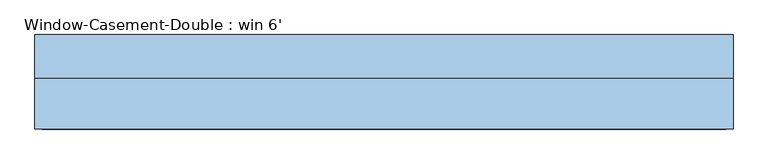
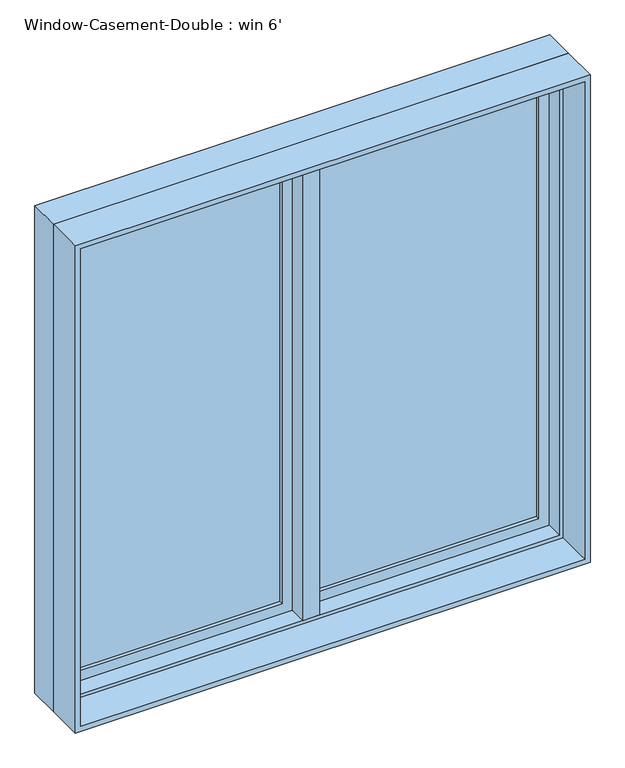
"""IFC4 building model written with IfcOpenShell, lengths in millimetres: window geometry, Window-Casement-Double : win 6'."""

from ifc_helpers import new_model, si_unit, frame, origin, place, context, project, spatial, polyline, outline, extrude, faceted_brep, source, transform, mapped, element, save


def window_casement_double_win_6_ce442eab(model_context):
    return source(origin(), model_context, "Body", "SolidModel", [
        faceted_brep([(9.525, 133.35, 2730.5), (-9.525, 133.35, 2730.5), (-9.525, 82.55, 2730.5), (9.525, 82.55, 2730.5), (9.525, 133.35, 927.1), (9.525, 82.55, 927.1), (-9.525, 82.55, 927.1), (-9.525, 133.35, 927.1), (-9.525, 82.55, 946.15), (-9.525, 82.55, 2711.45), (-30.1625, 82.55, 946.15), (-30.1625, 82.55, 2711.45), (-30.1625, 19.05, 946.15), (-30.1625, 19.05, 2711.45), (30.1625, 19.05, 946.15), (30.1625, 19.05, 2711.45), (30.1625, 82.55, 946.15), (30.1625, 82.55, 2711.45), (9.525, 82.55, 946.15), (9.525, 82.55, 2711.45)], [[[0, 1, 2, 3]], [[4, 5, 6, 7]], [[1, 0, 4, 7]], [[2, 1, 7, 6, 8, 9]], [[9, 8, 10, 11]], [[11, 10, 12, 13]], [[13, 12, 14, 15]], [[15, 14, 16, 17]], [[17, 16, 18, 19]], [[0, 3, 19, 18, 5, 4]], [[18, 8, 6, 5]], [[9, 19, 3, 2]], [[8, 18, 16, 14, 12, 10]], [[19, 9, 11, 13, 15, 17]]]),
        extrude(outline(polyline([(-66.675, 114.3), (-66.675, 107.95), (-844.55, 107.95), (-844.55, 114.3), (-66.675, 114.3)])), frame((0.0, 0.0, 984.25), z_axis=(0.0, 0.0, 1.0), x_axis=(1.0, 0.0, 0.0)), (0.0, 0.0, 1.0), 1689.1),
        extrude(outline(polyline([(-844.55, 95.25), (-844.55, 101.6), (-66.675, 101.6), (-66.675, 95.25), (-844.55, 95.25)])), frame((0.0, 0.0, 984.25), z_axis=(0.0, 0.0, 1.0), x_axis=(1.0, 0.0, 0.0)), (0.0, 0.0, 1.0), 1689.1),
        extrude(outline(polyline([(844.55, 114.3), (844.55, 107.95), (66.675, 107.95), (66.675, 114.3), (844.55, 114.3)])), frame((0.0, 0.0, 984.25), z_axis=(0.0, 0.0, 1.0), x_axis=(1.0, 0.0, 0.0)), (0.0, 0.0, 1.0), 1689.1),
        extrude(outline(polyline([(66.675, 95.25), (66.675, 101.6), (844.55, 101.6), (844.55, 95.25), (66.675, 95.25)])), frame((0.0, 0.0, 984.25), z_axis=(0.0, 0.0, 1.0), x_axis=(1.0, 0.0, 0.0)), (0.0, 0.0, 1.0), 1689.1),
        extrude(outline(polyline([(2730.5, -901.7), (927.1, -901.7), (927.1, -9.525), (2730.5, -9.525), (2730.5, -901.7)]), holes=[polyline([(2673.35, -66.675), (984.25, -66.675), (984.25, -844.55), (2673.35, -844.55), (2673.35, -66.675)])]), frame((0.0, 82.55, 0.0), z_axis=(0.0, 1.0, 0.0), x_axis=(0.0, 0.0, 1.0)), (0.0, 0.0, 1.0), 44.45),
        extrude(outline(polyline([(927.1, 901.7), (2730.5, 901.7), (2730.5, 9.525), (927.1, 9.525), (927.1, 901.7)]), holes=[polyline([(984.25, 66.675), (2673.35, 66.675), (2673.35, 844.55), (984.25, 844.55), (984.25, 66.675)])]), frame((0.0, 82.55, 0.0), z_axis=(0.0, 1.0, 0.0), x_axis=(0.0, 0.0, 1.0)), (0.0, 0.0, 1.0), 44.45),
        extrude(outline(polyline([(2743.2, -914.4), (914.4, -914.4), (914.4, 914.4), (2743.2, 914.4), (2743.2, -914.4)]), holes=[polyline([(2724.15, 895.35), (933.45, 895.35), (933.45, -895.35), (2724.15, -895.35), (2724.15, 895.35)])]), frame((0.0, -114.3, 0.0), z_axis=(0.0, 1.0, 0.0), x_axis=(0.0, 0.0, 1.0)), (0.0, 0.0, 1.0), 133.35),
        faceted_brep([(882.65, 82.55, 2711.45), (882.65, 19.05, 2711.45), (-882.65, 19.05, 2711.45), (-882.65, 82.55, 2711.45), (901.7, 133.35, 2730.5), (901.7, 82.55, 2730.5), (-901.7, 82.55, 2730.5), (-901.7, 133.35, 2730.5), (914.4, 19.05, 2743.2), (914.4, 133.35, 2743.2), (-914.4, 133.35, 2743.2), (-914.4, 19.05, 2743.2), (-882.65, 19.05, 946.15), (-882.65, 82.55, 946.15), (-901.7, 82.55, 927.1), (-901.7, 133.35, 927.1), (-914.4, 133.35, 914.4), (-914.4, 19.05, 914.4), (882.65, 19.05, 946.15), (882.65, 82.55, 946.15), (901.7, 82.55, 927.1), (901.7, 133.35, 927.1), (914.4, 133.35, 914.4), (914.4, 19.05, 914.4)], [[[0, 1, 2, 3]], [[4, 5, 6, 7]], [[8, 9, 10, 11]], [[3, 2, 12, 13]], [[7, 6, 14, 15]], [[11, 10, 16, 17]], [[13, 12, 18, 19]], [[15, 14, 20, 21]], [[17, 16, 22, 23]], [[11, 17, 23, 8], [1, 18, 12, 2]], [[19, 18, 1, 0]], [[5, 20, 14, 6], [3, 13, 19, 0]], [[21, 20, 5, 4]], [[23, 22, 9, 8]], [[9, 22, 16, 10], [7, 15, 21, 4]]]),
    ])


if __name__ == "__main__":
    model = new_model("IFC4")
    model_context = context("Model", 3, world=origin())
    ifc_project = project(units=[si_unit("LENGTHUNIT", "METRE", prefix="MILLI")], contexts=[model_context])
    site = spatial("IfcSite", under=ifc_project)
    building = spatial("IfcBuilding", under=site)
    placement = place(None, origin())
    window_casement_double_win_6_shape = window_casement_double_win_6_ce442eab(model_context)
    element("IfcWindow", 1, ObjectType="Window-Casement-Double : win 6'", at=placement, inside=building, context=model_context, shape_type="MappedRepresentation", body=[
        mapped(window_casement_double_win_6_shape, transform((0.0, 0.0, 0.0), x_axis=(1.0, 0.0, 0.0), y_axis=(0.0, 1.0, 0.0), z_axis=(0.0, 0.0, 1.0))),
    ])
    save(model, "model.ifc")

# Revit data of these elements
# Type "Window-Casement-Double : win 6'"
#   Type Mark = "18"
#   Fire Rating = "0.5h"
#   Assembly Code = "B2020100"
#   Analytic Construction = "Double glazing - domestic"
#   Frame Extension [instance default] = 0' - 0 1/4"
#   Window Inset [instance default] = 0' - 0"
#   Wall Thickness [instance default] = 0' - 6"
#   Interior Wall Closure [instance default] = 0' - 2 1/4"
#   Half Width = 3' - 0"
#   Visual Light Transmittance = 0.81
#   Thermal Resistance (R) = 1.8146 (h·ft²·°F)/BTU
#   Solar Heat Gain Coefficient = 0.76
#   Rough Width = 6' - 0 1/2"
#   Rough Height = 6' - 0 1/2"
#   Height = 6' - 0"
#   Heat Transfer Coefficient (U) = 0.5511 BTU/(h·ft²·°F)
#   Exterior Wall Closure [instance default] = 0' - 1 1/4"
#   Extension Jamb [instance default] = 0' - 2 1/4"
#   Default Sill Height = 3' - 0"
#   Width = 6' - 0"
#   Muntin Visibility = yes
#   Interior Trim Visibility [instance default] = yes
#   Exterior Trim Visibility [instance default] = yes
#   Extension Jamb Visibility [instance default] = yes
#   Interior Trim Material = Wood - Stained
#   Muntin Pattern = Muntin Pattern_2x2 : Muntin Pattern_2x2
#   Interior Trim = Trim-Window-Interior-Flat : Picture Frame
#   Interior Frame Material = Wood - Stained
#   Glass Panel Material = Glass
#   Exterior Trim Material = Clad - White
#   Exterior Trim = Trim-Window-Exterior-Flat : with Sill
#   Exterior Frame Material = Clad - White
#   Wall Closure = (empty or 0)
# Element 1 (IfcWindow, "Window-Casement-Double : win 6'")
#   Wall Thickness = 0' - 9"
#   Extension Jamb = 0' - 5 1/4"
#   Materials on its faces: "Wood - Stained", "Glass", "Clad - White"
# Materials
#   "Wood - Stained": class "Wood", colour RGB 224 178 126, transparency 0, Cost = 0
#   "Glass": class "Glass", colour RGB 0 128 192, transparency 0.75, Description = "Soda Lime Glass", Cost = 0
#   "Clad - White": class "Wood", colour RGB 242 242 238, transparency 0, Cost = 0
